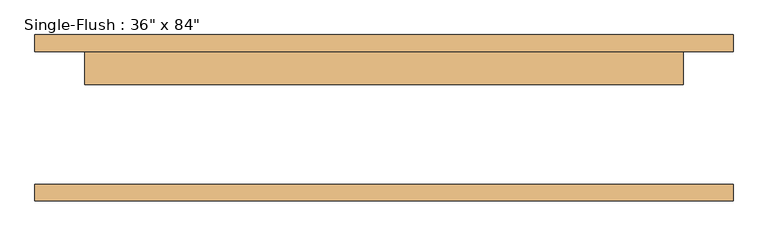
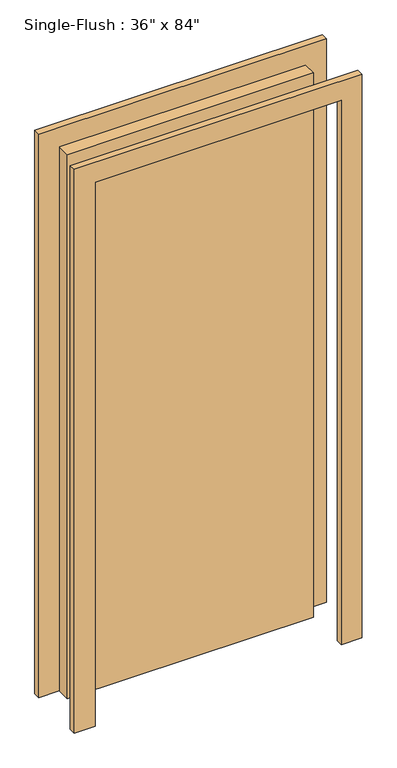
"""IFC4 building model written with IfcOpenShell, lengths in millimetres: door geometry."""

from ifc_helpers import new_model, si_unit, frame, origin, origin_with_axes, place, context, project, spatial, polyline, outline, extrude, source, transform, mapped, element, save


def door_54dd4da4(model_context):
    return source(origin(), model_context, "Body", "SweptSolid", [
        extrude(outline(polyline([(2209.8, -533.4), (0.0, -533.4), (0.0, -457.2), (2133.6, -457.2), (2133.6, 457.2), (0.0, 457.2), (0.0, 533.4), (2209.8, 533.4), (2209.8, -533.4)])), frame((0.0, 101.6, 0.0), z_axis=(0.0, 1.0, 0.0), x_axis=(0.0, 0.0, 1.0)), (0.0, 0.0, 1.0), 25.4),
        extrude(outline(polyline([(2209.8, 533.4), (2209.8, -533.4), (0.0, -533.4), (0.0, -457.2), (2133.6, -457.2), (2133.6, 457.2), (0.0, 457.2), (0.0, 533.4), (2209.8, 533.4)])), frame((0.0, -127.0, 0.0), z_axis=(0.0, 1.0, 0.0), x_axis=(0.0, 0.0, 1.0)), (0.0, 0.0, 1.0), 25.4),
        extrude(outline(polyline([(457.2, 50.8), (-457.2, 50.8), (-457.2, 101.6), (457.2, 101.6), (457.2, 50.8)])), origin_with_axes(), (0.0, 0.0, 1.0), 2133.6),
    ])


if __name__ == "__main__":
    model = new_model("IFC4")
    model_context = context("Model", 3, world=origin())
    ifc_project = project(units=[si_unit("LENGTHUNIT", "METRE", prefix="MILLI")], contexts=[model_context])
    site = spatial("IfcSite", under=ifc_project)
    building = spatial("IfcBuilding", under=site)
    placement = place(None, origin())
    door_shape = door_54dd4da4(model_context)
    element("IfcDoor", 1, ObjectType="Single-Flush : 36\" x 84\"", at=placement, inside=building, context=model_context, shape_type="MappedRepresentation", body=[
        mapped(door_shape, transform((0.0, 0.0, 0.0), x_axis=(1.0, 0.0, 0.0), y_axis=(0.0, 1.0, 0.0), z_axis=(0.0, 0.0, 1.0))),
    ])
    save(model, "model.ifc")

# Revit data of these elements
# Type "Single-Flush : 36\" x 84\""
#   Type Mark = "1"
#   Construction Type Id = "MDOOR"
#   Assembly Code = "C1020"
#   Analytic Construction = "Metal"
#   Thickness = 0' - 2"
#   Heat Transfer Coefficient (U) = 0.651978 BTU/(h·ft²·°F)
#   Height = 7' - 0"
#   Trim Projection Ext = 0' - 1"
#   Trim Projection Int = 0' - 1"
#   Trim Width = 0' - 3"
#   Width = 3' - 0"
#   Define Thermal Properties by = 1
#   Door Material = Door - Panel
#   Frame Material = Door - Frame
#   Visual Light Transmittance = 0
#   Solar Heat Gain Coefficient = 0
#   Function = (empty or 0)
#   Wall Closure = (empty or 0)
# Element 1 (IfcDoor, "Single-Flush : 36\" x 84\"")
#   Materials on its faces: "Door - Frame", "Door - Panel"
# Materials
#   "Door - Panel": class "Wood", colour RGB 210 159 95, transparency 0
#   "Door - Frame": colour RGB 118 70 51, transparency 0
